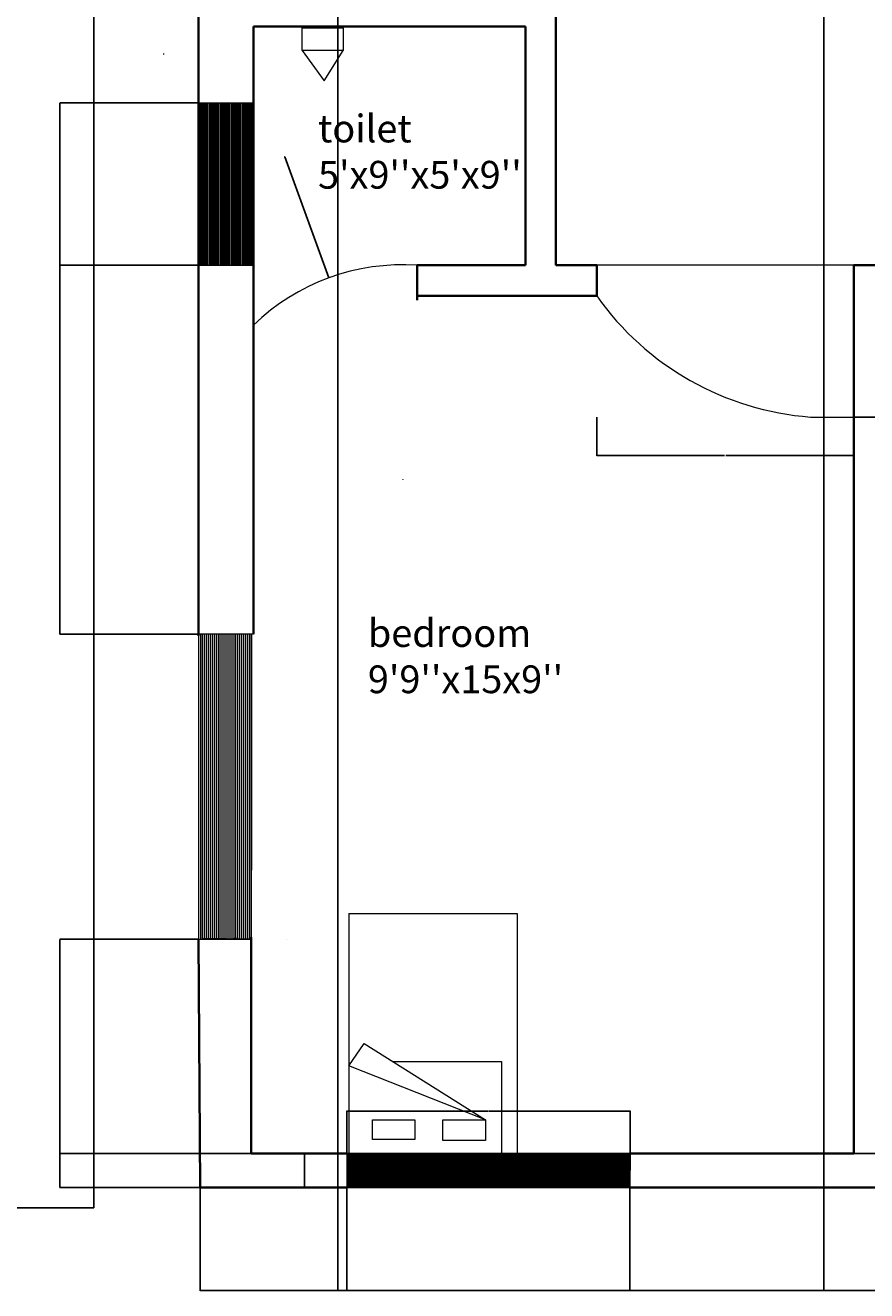
# Model space of a CAD drawing. Units: millimetres. Extents: x 1942 to 12281, y -2698 to 3078.
# Tile 4 of 6: x 6981 to 9104, y -2646 to 547. Entities that reach past the tile are written whole.
import ezdxf

# ---------------------------------------------------------------- set-up
doc = ezdxf.new("R2010")
doc.units = ezdxf.units.MM
for name, color, linetype, lineweight in [('A-ANNO-DIMS', 2, 'Continuous', 18), ('A-AREA-IDEN', 3, 'Continuous', 18), ('A-DETL-REF', 8, 'Continuous', 13), ('A-DOOR', 4, 'Continuous', 18), ('A-FLOR-FIXT', 9, 'Continuous', 18), ('A-FURN', 8, 'Continuous', 18), ('A-GLAZ', 4, 'Continuous', 18), ('A-GLAZ-PATT', 9, 'Continuous', 13), ('A-WALL', 7, 'Continuous', 35)]:
    doc.layers.add(name, color=color, linetype=linetype, lineweight=lineweight)
doc.styles.get("Standard").update_dxf_attribs({"font": 'arial.ttf'})
doc.dimstyles.get("Standard").update_dxf_attribs({"dimtxt": 0.18, "dimasz": 0.18, "dimexe": 0.18, "dimexo": 0.0625, "dimgap": 0.09, "dimtad": 0, "dimtih": 1, "dimtoh": 1, "dimdec": 4, "dimzin": 0, "dimdsep": 46, "dimtxsty": 'Standard', "dimcen": 0.09, "dimadec": 0, "dimazin": 0, "dimtfac": 1, "dimtdec": 4, "dimtofl": 0, "dimtmove": 0, "dimatfit": 3, "dimfxl": 1, "dimtolj": 1, "dimtzin": 0, "dimarcsym": 0})

# ---------------------------------------------------------------- blocks, each defined once
blk = doc.blocks.new('BED-PILLOWS')
for p, q in [((0, 605.9), (424.9, 605.9)), ((0, 605.9), (0, 0)), ((424.9, 605.9), (424.9, 0)), ((0, 221), (38.1, 277.4)), ((38.1, 277.4), (344.8, 84.6)), ((109.8, 232.4), (384.7, 232.4)), ((384.7, 232.4), (384.7, 0)), ((344.8, 84.6), (0, 221)), ((0, 0), (0, 0))]:
    blk.add_line(p, q)
for points in [[(59.7, 84.6), (166.4, 84.6), (166.4, 35.4), (59.7, 35.4)], [(236.8, 84.6), (344.8, 84.6), (344.8, 33.1), (236.8, 33.1)]]:
    blk.add_lwpolyline(points, close=True)
blk = doc.blocks.new('WC-TAPERED-LONG')
for p, q in [((0, 77), (55.9, 0)), ((55.9, 0), (103.2, 77))]:
    blk.add_line(p, q)
blk.add_lwpolyline([(0, 134), (103.2, 134), (103.2, 77), (0, 77)], close=True)
blk = doc.blocks.new('DOOR-BEDROOM')
for p, q in [((648.7, 382.9), (0, 382.9)), ((539.8, 0), (648.7, 0))]:
    blk.add_line(p, q)
blk.add_arc((594.3, 726.1), 728.1, 215.2982, 265.7132)
blk = doc.blocks.new('DOOR-WC-BEDROOM')
blk.add_arc((376.5, -390), 542.1, 86.1851, 133.9877)
blk = doc.blocks.new('WIN-BEDROOM-SIDE')
for p, q in [((138.7, 769.7), (0, 769.7)), ((132.6, 771), (132.6, 5.6)), ((0, 765.5), (0, 0.1)), ((0, 0.1), (132.6, 0.1)), ((8.8, 3.3), (132.6, 1.4)), ((95.6, 3.3), (78.2, 0))]:
    blk.add_line(p, q)
blk = doc.blocks.new('WIN-BEDROOM-END')
for p, q in [((0, 85.7), (0, 0)), ((0, 85.7), (430, 85.7)), ((714.9, 85.7), (714.3, 0)), ((714.3, 0), (1.8, 0))]:
    blk.add_line(p, q)
blk = doc.blocks.new('*D38')
at = {"layer": 'A-ANNO-DIMS', "color": 0, "lineweight": -2, "transparency": 16777216}
for p, q in [((8423.1, -441.8), (8423.1, -539.2)), ((9071.8, -441.8), (9071.8, -539.2)), ((8423.3, -539), (8745.8, -539)), ((9071.6, -539), (8749.1, -539))]:
    blk.add_line(p, q, dxfattribs=at)
at = {"layer": 'A-ANNO-DIMS', "color": 0, "transparency": 16777216}
for points in [[(8423.3, -539), (8423.3, -539.1), (8423.1, -539)], [(9071.6, -539), (9071.6, -539.1), (9071.8, -539)]]:
    blk.add_solid(points, dxfattribs=at)
at = {"layer": 'Defpoints', "color": 0, "transparency": 16777216}
for p in [(8423.1, -441.7), (9071.8, -441.7), (9071.8, -539)]:
    blk.add_point(p, dxfattribs=at)
at = {"layer": 'A-ANNO-DIMS', "color": 0, "transparency": 16777216, "insert": (8747.4, -539), "char_height": 0.18, "attachment_point": 5}
blk.add_mtext('\\A1;BEDROOM DOOR 649 TYP.', dxfattribs=at)
blk = doc.blocks.new('*D39')
at = {"layer": 'A-ANNO-DIMS', "color": 0, "lineweight": -2, "transparency": 16777216}
for p, q in [((9071.9, -58.9), (9169.3, -58.9)), ((9169.1, -59), (9169.1, -250.1)), ((9169.1, -441.5), (9169.1, -250.5)), ((9071.9, -441.7), (9169.3, -441.7))]:
    blk.add_line(p, q, dxfattribs=at)
at = {"layer": 'A-ANNO-DIMS', "color": 0, "transparency": 16777216}
for points in [[(9169.1, -59), (9169.1, -59), (9169.1, -58.9)], [(9169.1, -441.5), (9169.1, -441.5), (9169.1, -441.7)]]:
    blk.add_solid(points, dxfattribs=at)
at = {"layer": 'Defpoints', "color": 0, "transparency": 16777216}
for p in [(9071.8, -58.9), (9169.1, -58.9), (9071.8, -441.7)]:
    blk.add_point(p, dxfattribs=at)
at = {"layer": 'A-ANNO-DIMS', "color": 0, "transparency": 16777216, "insert": (9169.1, -250.3), "char_height": 0.18, "attachment_point": 5}
blk.add_mtext('\\A1;383 TYP.', dxfattribs=at)
blk = doc.blocks.new('*D66')
at = {"layer": 'A-ANNO-DIMS', "color": 0, "lineweight": -2, "transparency": 16777216}
for p, q in [((7792.8, -2299.7), (7792.8, -2192.4)), ((7793, -2192.6), (8149.5, -2192.6)), ((8507.6, -2192.6), (8151.1, -2192.6)), ((8507.7, -2299.7), (8507.7, -2192.4))]:
    blk.add_line(p, q, dxfattribs=at)
at = {"layer": 'A-ANNO-DIMS', "color": 0, "transparency": 16777216}
for points in [[(7793, -2192.5), (7793, -2192.6), (7792.8, -2192.6)], [(8507.6, -2192.5), (8507.6, -2192.6), (8507.7, -2192.6)]]:
    blk.add_solid(points, dxfattribs=at)
at = {"layer": 'Defpoints', "color": 0, "transparency": 16777216}
for p in [(8507.7, -2192.6), (7792.8, -2299.8), (8507.7, -2299.8)]:
    blk.add_point(p, dxfattribs=at)
at = {"layer": 'A-ANNO-DIMS', "color": 0, "transparency": 16777216, "insert": (8150.3, -2192.6), "char_height": 0.18, "attachment_point": 5}
blk.add_mtext('\\A1;W4 715 TYP.', dxfattribs=at)
blk = doc.blocks.new('*D67')
at = {"layer": 'A-ANNO-DIMS', "color": 0, "lineweight": -2, "transparency": 16777216}
for p, q in [((7792.8, -2299.8), (7685.4, -2299.8)), ((7685.6, -2300), (7685.6, -2342.5)), ((7685.6, -2385.3), (7685.6, -2342.8)), ((7792.8, -2385.5), (7685.4, -2385.5))]:
    blk.add_line(p, q, dxfattribs=at)
at = {"layer": 'A-ANNO-DIMS', "color": 0, "transparency": 16777216}
for points in [[(7685.6, -2300), (7685.6, -2300), (7685.6, -2299.8)], [(7685.6, -2385.3), (7685.6, -2385.3), (7685.6, -2385.5)]]:
    blk.add_solid(points, dxfattribs=at)
at = {"layer": 'Defpoints', "color": 0, "transparency": 16777216}
for p in [(7685.6, -2299.8), (7792.8, -2299.8), (7792.8, -2385.5)]:
    blk.add_point(p, dxfattribs=at)
at = {"layer": 'A-ANNO-DIMS', "color": 0, "transparency": 16777216, "insert": (7685.6, -2342.6), "char_height": 0.18, "attachment_point": 5}
blk.add_mtext('\\A1;86 TYP.', dxfattribs=at)
blk = doc.blocks.new('*D71')
at = {"layer": 'A-ANNO-DIMS', "color": 0, "lineweight": -2, "transparency": 16777216}
for p, q in [((6894.2, 2765.9), (7154.5, 2765.9)), ((7154.3, 2765.7), (7154.3, 164.5)), ((7154.3, -2437.1), (7154.3, 164.1)), ((6894.2, -2437.2), (7154.5, -2437.2))]:
    blk.add_line(p, q, dxfattribs=at)
at = {"layer": 'A-ANNO-DIMS', "color": 0, "transparency": 16777216}
for points in [[(7154.3, 2765.7), (7154.4, 2765.7), (7154.3, 2765.9)], [(7154.3, -2437.1), (7154.4, -2437.1), (7154.3, -2437.2)]]:
    blk.add_solid(points, dxfattribs=at)
at = {"layer": 'Defpoints', "color": 0, "transparency": 16777216}
for p in [(6894.1, 2765.9), (7154.3, 2765.9), (6894.1, -2437.2)]:
    blk.add_point(p, dxfattribs=at)
at = {"layer": 'A-ANNO-DIMS', "color": 0, "transparency": 16777216, "insert": (7154.3, 164.3), "char_height": 0.18, "attachment_point": 5}
blk.add_mtext('\\A1;5203', dxfattribs=at)
blk = doc.blocks.new('*D95')
at = {"layer": 'A-ANNO-DIMS', "color": 0, "lineweight": -2, "transparency": 16777216}
for p, q in [((7422.1, -2385.6), (7422.1, -2645.9)), ((7792.8, -2385.6), (7792.8, -2645.9)), ((7422.3, -2645.7), (7607.1, -2645.7)), ((7792.7, -2645.7), (7607.9, -2645.7))]:
    blk.add_line(p, q, dxfattribs=at)
at = {"layer": 'A-ANNO-DIMS', "color": 0, "transparency": 16777216}
for points in [[(7422.3, -2645.7), (7422.3, -2645.7), (7422.1, -2645.7)], [(7792.7, -2645.7), (7792.7, -2645.7), (7792.8, -2645.7)]]:
    blk.add_solid(points, dxfattribs=at)
at = {"layer": 'Defpoints', "color": 0, "transparency": 16777216}
for p in [(7422.1, -2385.5), (7792.8, -2385.5), (7792.8, -2645.7)]:
    blk.add_point(p, dxfattribs=at)
at = {"layer": 'A-ANNO-DIMS', "color": 0, "transparency": 16777216, "insert": (7607.5, -2645.7), "char_height": 0.18, "attachment_point": 5}
blk.add_mtext('\\A1;370.7', dxfattribs=at)
blk = doc.blocks.new('*D96')
at = {"layer": 'A-ANNO-DIMS', "color": 0, "lineweight": -2, "transparency": 16777216}
for p, q in [((8507.1, -2385.6), (8507.1, -2645.9)), ((9137.2, -2385.6), (9137.2, -2645.9)), ((8507.3, -2645.7), (8821.8, -2645.7)), ((9137, -2645.7), (8822.5, -2645.7))]:
    blk.add_line(p, q, dxfattribs=at)
at = {"layer": 'A-ANNO-DIMS', "color": 0, "transparency": 16777216}
for points in [[(8507.3, -2645.7), (8507.3, -2645.7), (8507.1, -2645.7)], [(9137, -2645.7), (9137, -2645.7), (9137.2, -2645.7)]]:
    blk.add_solid(points, dxfattribs=at)
at = {"layer": 'Defpoints', "color": 0, "transparency": 16777216}
for p in [(8507.1, -2385.5), (9137.2, -2385.5), (9137.2, -2645.7)]:
    blk.add_point(p, dxfattribs=at)
at = {"layer": 'A-ANNO-DIMS', "color": 0, "transparency": 16777216, "insert": (8822.1, -2645.7), "char_height": 0.18, "attachment_point": 5}
blk.add_mtext('\\A1;630.1', dxfattribs=at)
blk = doc.blocks.new('*D97')
at = {"layer": 'A-ANNO-DIMS', "color": 0, "lineweight": -2, "transparency": 16777216}
for p, q in [((7418.5, -1759.3), (7068.5, -1759.3)), ((7068.7, -1759.5), (7068.7, -2072.2)), ((7068.7, -2385.3), (7068.7, -2072.6)), ((7422.1, -2385.5), (7068.5, -2385.5))]:
    blk.add_line(p, q, dxfattribs=at)
at = {"layer": 'A-ANNO-DIMS', "color": 0, "transparency": 16777216}
for points in [[(7068.7, -1759.5), (7068.8, -1759.5), (7068.7, -1759.3)], [(7068.7, -2385.3), (7068.8, -2385.3), (7068.7, -2385.5)]]:
    blk.add_solid(points, dxfattribs=at)
at = {"layer": 'Defpoints', "color": 0, "transparency": 16777216}
for p in [(7068.7, -1759.3), (7418.5, -1759.3), (7422.1, -2385.5)]:
    blk.add_point(p, dxfattribs=at)
at = {"layer": 'A-ANNO-DIMS', "color": 0, "transparency": 16777216, "insert": (7068.7, -2072.4), "char_height": 0.18, "attachment_point": 5}
blk.add_mtext('\\A1;626.2', dxfattribs=at)
blk = doc.blocks.new('*D98')
at = {"layer": 'A-ANNO-DIMS', "color": 0, "lineweight": -2, "transparency": 16777216}
for p, q in [((7418.5, -58.9), (7068.5, -58.9)), ((7068.7, -59), (7068.7, -524.1)), ((7068.7, -989.6), (7068.7, -524.5)), ((7418.5, -989.8), (7068.5, -989.8))]:
    blk.add_line(p, q, dxfattribs=at)
at = {"layer": 'A-ANNO-DIMS', "color": 0, "transparency": 16777216}
for points in [[(7068.7, -59), (7068.8, -59), (7068.7, -58.9)], [(7068.7, -989.6), (7068.8, -989.6), (7068.7, -989.8)]]:
    blk.add_solid(points, dxfattribs=at)
at = {"layer": 'Defpoints', "color": 0, "transparency": 16777216}
for p in [(7068.7, -58.9), (7418.5, -58.9), (7418.5, -989.8)]:
    blk.add_point(p, dxfattribs=at)
at = {"layer": 'A-ANNO-DIMS', "color": 0, "transparency": 16777216, "insert": (7068.7, -524.3), "char_height": 0.18, "attachment_point": 5}
blk.add_mtext('\\A1;931', dxfattribs=at)
blk = doc.blocks.new('*D99')
at = {"layer": 'A-ANNO-DIMS', "color": 0, "lineweight": -2, "transparency": 16777216}
for p, q in [((7418.5, 350.6), (7068.5, 350.6)), ((7068.7, 350.4), (7068.7, 146.1)), ((7068.7, -58.7), (7068.7, 145.7)), ((7418.5, -58.9), (7068.5, -58.9))]:
    blk.add_line(p, q, dxfattribs=at)
at = {"layer": 'A-ANNO-DIMS', "color": 0, "transparency": 16777216}
for points in [[(7068.7, 350.4), (7068.8, 350.4), (7068.7, 350.6)], [(7068.7, -58.7), (7068.8, -58.7), (7068.7, -58.9)]]:
    blk.add_solid(points, dxfattribs=at)
at = {"layer": 'Defpoints', "color": 0, "transparency": 16777216}
for p in [(7068.7, 350.6), (7418.5, 350.6), (7418.5, -58.9)]:
    blk.add_point(p, dxfattribs=at)
at = {"layer": 'A-ANNO-DIMS', "color": 0, "transparency": 16777216, "insert": (7068.7, 145.9), "char_height": 0.18, "attachment_point": 5}
blk.add_mtext('\\A1;409.45', dxfattribs=at)
blk = doc.blocks.new('*D105')
at = {"layer": 'A-ANNO-DIMS', "color": 0, "lineweight": -2, "transparency": 16777216}
for p, q in [((7769.8, 1304.1), (7769.8, -2645.9)), ((8996.6, 1304.1), (8996.6, -2645.9)), ((7770, -2645.7), (8382.7, -2645.7)), ((8996.4, -2645.7), (8383.6, -2645.7))]:
    blk.add_line(p, q, dxfattribs=at)
at = {"layer": 'A-ANNO-DIMS', "color": 0, "transparency": 16777216}
for points in [[(7770, -2645.7), (7770, -2645.7), (7769.8, -2645.7)], [(8996.4, -2645.7), (8996.4, -2645.7), (8996.6, -2645.7)]]:
    blk.add_solid(points, dxfattribs=at)
at = {"layer": 'Defpoints', "color": 0, "transparency": 16777216}
for p in [(7769.8, 1304.1), (8996.6, 1304.1), (8996.6, -2645.7)]:
    blk.add_point(p, dxfattribs=at)
at = {"layer": 'A-ANNO-DIMS', "color": 0, "transparency": 16777216, "insert": (8383.2, -2645.7), "char_height": 0.18, "attachment_point": 5}
blk.add_mtext('\\A1;1226.8', dxfattribs=at)
blk = doc.blocks.new('*D113')
at = {"layer": 'A-ANNO-DIMS', "color": 0, "lineweight": -2, "transparency": 16777216}
for p, q in [((11807.9, -2299.8), (7068.5, -2299.8)), ((7068.7, -2300), (7068.7, -2342.5)), ((7068.7, -2385.3), (7068.7, -2342.8)), ((12020.5, -2385.5), (7068.5, -2385.5))]:
    blk.add_line(p, q, dxfattribs=at)
at = {"layer": 'A-ANNO-DIMS', "color": 0, "transparency": 16777216}
for points in [[(7068.7, -2300), (7068.8, -2300), (7068.7, -2299.8)], [(7068.7, -2385.3), (7068.8, -2385.3), (7068.7, -2385.5)]]:
    blk.add_solid(points, dxfattribs=at)
at = {"layer": 'Defpoints', "color": 0, "transparency": 16777216}
for p in [(11807.9, -2299.8), (7068.7, -2385.5), (12020.6, -2385.5)]:
    blk.add_point(p, dxfattribs=at)
at = {"layer": 'A-ANNO-DIMS', "color": 0, "transparency": 16777216, "insert": (7068.7, -2342.6), "char_height": 0.18, "attachment_point": 5}
blk.add_mtext('\\A1;85.68', dxfattribs=at)
blk = doc.blocks.new('*D116')
at = {"layer": 'A-ANNO-DIMS', "color": 0, "lineweight": -2, "transparency": 16777216}
for p, q in [((7635.6, 214.8), (7635.8, 214.8)), ((7635.8, 214.8), (7747.4, -90.5)), ((7933.6, -599.7), (7933.8, -599.7)), ((7933.7, -599.8), (7933.7, -599.7))]:
    blk.add_line(p, q, dxfattribs=at)
at = {"layer": 'A-ANNO-DIMS', "color": 0, "transparency": 16777216}
blk.add_solid([(7747.5, -90.4), (7747.4, -90.5), (7747.5, -90.6)], dxfattribs=at)
at = {"layer": 'Defpoints', "color": 0, "transparency": 16777216}
for p in [(7747.5, -90.6), (7933.7, -599.7)]:
    blk.add_point(p, dxfattribs=at)
at = {"layer": 'A-ANNO-DIMS', "color": 0, "transparency": 16777216, "insert": (7635, 214.8), "char_height": 0.18, "attachment_point": 5}
blk.add_mtext('\\A1;2X R542.1', dxfattribs=at)

msp = doc.modelspace()

# ---------------------------------------------------------------- hatches: boundary and pattern name
at = {"layer": 'A-GLAZ-PATT'}
h = msp.add_hatch(dxfattribs=at)
h.set_pattern_fill('ANSI31', color=256, scale=1.091886, angle=45, style=0)
h.paths.add_polyline_path([(7418.529, -58.855), (7557.198, -58.855), (7557.198, 350.597), (7418.529, 350.597)])
h = msp.add_hatch(dxfattribs=at)
h.set_pattern_fill('ANSI31', color=256, scale=1.559837, angle=45, style=0)
h.paths.add_polyline_path([(7418.529, -1759.33), (7551.172, -1759.33), (7557.198, -989.765), (7418.529, -989.765)])
h = msp.add_hatch(dxfattribs=at)
h.set_pattern_fill('ANSI31', color=256, scale=0.870611, angle=135, style=0)
h.paths.add_polyline_path([(7792.843, -2385.489), (8507.109, -2385.489), (8507.74, -2299.801), (7792.843, -2299.799)])

# ---------------------------------------------------------------- linework, layer by layer
at = {"layer": 'A-DETL-REF'}
for p, q in [((7331.428, 474.017), (7328.928, 474.017)), ((7639.851, -1759.33), (7639.851, -1759.33))]:
    msp.add_line(p, q, dxfattribs=at)
at = {"layer": 'A-GLAZ'}
for p, q in [((7418.529, 350.597), (7557.198, 350.597)), ((7418.529, -58.855), (7557.198, -58.855))]:
    msp.add_line(p, q, dxfattribs=at)
at = {"layer": 'A-WALL'}
for p, q in [((8320.239, 821.112), (8320.239, 96.726)), ((7418.529, 793.021), (7418.529, 350.597)), ((7557.198, 350.597), (7557.198, 543.943)), ((7557.198, 543.943), (7778.589, 543.943)), ((7778.589, 543.943), (8094.415, 543.943)), ((8094.415, 543.943), (8243.328, 543.943)), ((8243.328, 543.943), (8243.328, 90.185)), ((7418.529, 350.597), (7418.529, 350.597)), ((7418.529, 350.597), (7418.529, -993.969)), ((7557.198, 350.597), (7557.198, -989.765)), ((8320.239, 96.726), (8320.239, -58.855)), ((8243.328, 90.185), (8243.328, -58.855)), ((7969.747, -58.855), (8243.328, -58.855)), ((7969.747, -58.855), (7969.747, -146.751)), ((8320.239, -58.855), (8423.103, -58.855)), ((8423.103, -58.855), (8423.103, -58.855)), ((8423.103, -58.855), (8423.103, -136.375)), ((9071.789, -965.418), (9071.789, -58.855)), ((9071.789, -58.855), (9137.19, -58.855)), ((8423.103, -136.375), (7969.747, -136.375)), ((9071.789, -2299.81), (9071.789, -965.418)), ((7551.172, -1753.808), (7551.172, -2299.799)), ((7418.529, -1759.33), (7422.136, -2385.489)), ((7551.172, -2299.799), (7792.843, -2299.799)), ((8507.74, -2299.801), (9071.789, -2299.81)), ((7422.136, -2385.489), (7794.593, -2385.489)), ((8507.109, -2385.489), (9137.19, -2385.489))]:
    msp.add_line(p, q, dxfattribs=at)

# ---------------------------------------------------------------- block references
at = {"layer": 'A-DOOR'}
for name, p in [('DOOR-WC-BEDROOM', (7557.198, -209.716)), ('DOOR-BEDROOM', (8423.102, -441.726))]:
    msp.add_blockref(name, p, dxfattribs=at)
at = {"layer": 'A-FLOR-FIXT'}
msp.add_blockref('WC-TAPERED-LONG', (7679.918, 406.26), dxfattribs=at)
at = {"layer": 'A-FURN'}
msp.add_blockref('BED-PILLOWS', (7797.894, -2299.799), dxfattribs=at)
at = {"layer": 'A-GLAZ'}
for name, p in [('WIN-BEDROOM-SIDE', (7418.529, -1759.452)), ('WIN-BEDROOM-END', (7792.843, -2385.489))]:
    msp.add_blockref(name, p, dxfattribs=at)

# ---------------------------------------------------------------- texts
at = {"layer": 'A-AREA-IDEN', "insert": (7720.012, 321.142), "char_height": 70, "attachment_point": 1}
msp.add_mtext_dynamic_manual_height_columns("{toilet\\P5'x9''x5'x9''}", width=77.58841, gutter_width=12.5, heights=[0], dxfattribs=at)
at = {"layer": 'A-AREA-IDEN', "insert": (7845.712, -951.746), "char_height": 70, "attachment_point": 1}
msp.add_mtext("{bedroom\\P9'9''x15x9''}", dxfattribs=at)

# ---------------------------------------------------------------- dimensions: what is measured, and where the dimension line sits
at = {"layer": 'A-ANNO-DIMS'}
for base, p1, p2, override, picture, middle in [((7154.346, 2765.873), (6894.096, -2437.233), (6894.096, 2765.873), {"dimdec": 0, "dimlfac": 1, "dimrnd": 0, "dimzin": 0, "dimdsep": 46, "dimlunit": 2}, '*D71', (7154.346, 164.32)), ((7068.728, 350.597), (7418.529, -58.855), (7418.529, 350.597), {"dimdec": 2, "dimlfac": 1, "dimrnd": 0, "dimzin": 0, "dimdsep": 46, "dimlunit": 2}, '*D99', (7068.728, 145.871)), ((7068.728, -58.855), (7418.529, -989.765), (7418.529, -58.855), {"dimdec": 0, "dimlfac": 1, "dimrnd": 0, "dimzin": 0, "dimdsep": 46, "dimlunit": 2}, '*D98', (7068.728, -524.31)), ((7068.728, -1759.33), (7422.136, -2385.489), (7418.529, -1759.33), {"dimdec": 1, "dimlfac": 1, "dimrnd": 0, "dimzin": 0, "dimdsep": 46, "dimlunit": 2}, '*D97', (7068.728, -2072.41)), ((7068.728, -2385.489), (11807.937, -2299.81), (12020.574, -2385.489), {"dimdec": 2, "dimlfac": 1, "dimrnd": 0, "dimzin": 0, "dimdsep": 46, "dimlunit": 2}, '*D113', (7068.728, -2342.65))]:
    dim = msp.add_linear_dim(base=base, p1=p1, p2=p2, angle=90, dimstyle='Standard', override=override, dxfattribs=at)
    dim.commit()
    dim.dimension.update_dxf_attribs({"geometry": picture, "text_midpoint": middle})
for base, p1, p2, picture, middle in [((8996.556, -2645.689), (7769.776, 1304.131), (8996.556, 1304.131), '*D105', (8383.166, -2645.689)), ((7792.843, -2645.689), (7422.136, -2385.489), (7792.843, -2385.489), '*D95', (7607.49, -2645.689)), ((9137.19, -2645.689), (8507.109, -2385.489), (9137.19, -2385.489), '*D96', (8822.15, -2645.689))]:
    dim = msp.add_linear_dim(base=base, p1=p1, p2=p2, dimstyle='Standard', override={"dimdec": 1, "dimlfac": 1, "dimrnd": 0, "dimzin": 0, "dimdsep": 46, "dimlunit": 2}, dxfattribs=at)
    dim.commit()
    dim.dimension.update_dxf_attribs({"geometry": picture, "text_midpoint": middle})
dim = msp.add_radius_dim(center=(7933.68, -599.74), mpoint=(7747.508, -90.626), text='2X <>', dimstyle='Standard', override={"dimdec": 1, "dimlfac": 1, "dimrnd": 0, "dimzin": 0, "dimdsep": 46, "dimlunit": 2}, dxfattribs=at)
dim.commit()
dim.dimension.update_dxf_attribs({"geometry": '*D116', "text_midpoint": (7634.968, 214.843), "dimtype": 164})
for base, p1, p2, picture, middle in [((9169.091, -58.855), (9071.789, -441.726), (9071.789, -58.855), '*D39', (9169.091, -250.291)), ((7685.609, -2299.799), (7792.843, -2385.489), (7792.843, -2299.799), '*D67', (7685.609, -2342.644))]:
    dim = msp.add_linear_dim(base=base, p1=p1, p2=p2, angle=90, text='<> TYP.', dimstyle='Standard', override={"dimdec": 0, "dimlfac": 1, "dimrnd": 0, "dimzin": 0, "dimdsep": 46, "dimlunit": 2}, dxfattribs=at)
    dim.commit()
    dim.dimension.update_dxf_attribs({"geometry": picture, "text_midpoint": middle})
for base, p1, p2, text, picture, middle in [((9071.789, -539.029), (8423.103, -441.726), (9071.789, -441.726), 'BEDROOM DOOR <> TYP.', '*D38', (8747.446, -539.029)), ((8507.74, -2192.565), (7792.843, -2299.799), (8507.74, -2299.799), 'W4 <> TYP.', '*D66', (8150.292, -2192.565))]:
    dim = msp.add_linear_dim(base=base, p1=p1, p2=p2, text=text, dimstyle='Standard', override={"dimdec": 0, "dimlfac": 1, "dimrnd": 0, "dimzin": 0, "dimdsep": 46, "dimlunit": 2}, dxfattribs=at)
    dim.commit()
    dim.dimension.update_dxf_attribs({"geometry": picture, "text_midpoint": middle})

doc.saveas('drawing.dxf')
